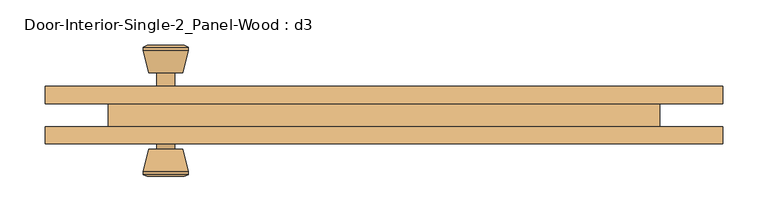
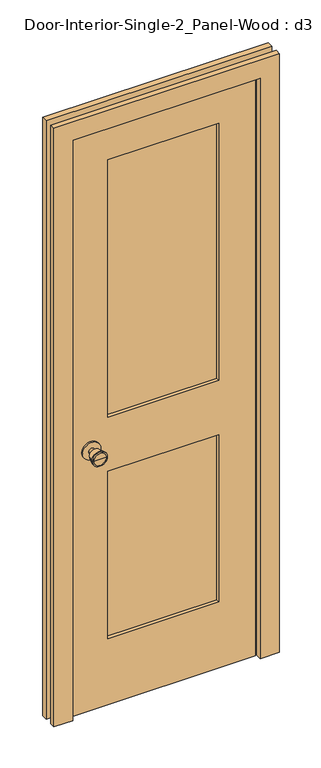
"""IFC4 building model written with IfcOpenShell, lengths in millimetres: door geometry, Door-Interior-Single-2_Panel-Wood : d3."""

from ifc_helpers import new_model, si_unit, point, frame, frame_2d, origin, place, context, project, spatial, polyline, circle_curve, trimmed, segment, composite_curve, outline, extrude, source, transform, mapped, element, save
from ifc_brep_helpers import plane_surface, cylinder_surface, revolved_surface, advanced_brep


def door_interior_single_2_panel_wood_d3_c9a7c184(model_context):
    return source(origin(), model_context, "Body", "SolidModel", [
        advanced_brep(
        [(-241.3, 31.4, 914.4), (-251.3, 31.4, 914.4), (-231.3, 31.4, 914.4), (-220.8241324, 80.4, 914.4), (-261.7758676, 80.4, 914.4), (-241.3, 80.4, 914.4), (-216.3, 78.5721319, 914.4), (-266.3, 78.5721319, 914.4), (-216.3, 75.1084537, 914.4), (-266.3, 75.1084537, 914.4), (-222.663764, 50.4, 914.4), (-259.936236, 50.4, 914.4), (-231.3, 50.4, 914.4), (-251.3, 50.4, 914.4)],
        [
            (0, 1),
            (1, 2, circle_curve(frame((-241.3, 31.4, 914.4), z_axis=(0.0, -1.0, 0.0), x_axis=(-1.0, 0.0, 0.0)), 10.0)),
            (2, 0),
            (2, 1, circle_curve(frame((-241.3, 31.4, 914.4), z_axis=(0.0, -1.0, 0.0), x_axis=(-1.0, 0.0, 0.0)), 10.0)),
            (3, 4, circle_curve(frame((-241.3, 80.4, 914.4), z_axis=(0.0, 1.0, 0.0), x_axis=(-1.0, 0.0, 0.0)), 20.4758676)),
            (4, 5),
            (5, 3),
            (4, 3, circle_curve(frame((-241.3, 80.4, 914.4), z_axis=(0.0, 1.0, 0.0), x_axis=(-1.0, 0.0, 0.0)), 20.4758676)),
            (6, 7, circle_curve(frame((-241.3, 78.5721319, 914.4), z_axis=(0.0, 1.0, 0.0), x_axis=(-1.0, 0.0, 0.0)), 25.0)),
            (7, 4),
            (3, 6),
            (7, 6, circle_curve(frame((-241.3, 78.5721319, 914.4), z_axis=(0.0, 1.0, 0.0), x_axis=(-1.0, 0.0, 0.0)), 25.0)),
            (8, 9, circle_curve(frame((-241.3, 75.1084537, 914.4), z_axis=(0.0, 1.0, 0.0), x_axis=(-1.0, 0.0, 0.0)), 25.0)),
            (9, 7),
            (6, 8),
            (9, 8, circle_curve(frame((-241.3, 75.1084537, 914.4), z_axis=(0.0, 1.0, 0.0), x_axis=(-1.0, 0.0, 0.0)), 25.0)),
            (10, 11, circle_curve(frame((-241.3, 50.4, 914.4), z_axis=(0.0, 1.0, 0.0), x_axis=(-1.0, 0.0, 0.0)), 18.636236)),
            (11, 9),
            (8, 10),
            (11, 10, circle_curve(frame((-241.3, 50.4, 914.4), z_axis=(0.0, 1.0, 0.0), x_axis=(-1.0, 0.0, 0.0)), 18.636236)),
            (12, 13, circle_curve(frame((-241.3, 50.4, 914.4), z_axis=(0.0, 1.0, 0.0), x_axis=(-1.0, 0.0, 0.0)), 10.0)),
            (13, 11),
            (10, 12),
            (13, 12, circle_curve(frame((-241.3, 50.4, 914.4), z_axis=(0.0, 1.0, 0.0), x_axis=(-1.0, 0.0, 0.0)), 10.0)),
            (1, 13),
            (12, 2),
        ],
        [
            plane_surface(frame((-241.3, 31.4, 914.4), z_axis=(0.0, -1.0, 0.0), x_axis=(-1.0, 0.0, 0.0))),
            plane_surface(frame((-241.3, 80.4, 914.4), z_axis=(0.0, 1.0, 0.0), x_axis=(-1.0, 0.0, 0.0))),
            revolved_surface(polyline([(-261.7758676, 80.4, 914.4), (-266.3, 78.5721319, 914.4)]), (-241.3, 31.4, 914.4), (0.0, -1.0, 0.0)),
            cylinder_surface(frame((-241.3, 31.4, 914.4), z_axis=(0.0, -1.0, 0.0), x_axis=(-1.0, 0.0, 0.0)), 25.0),
            revolved_surface(polyline([(-266.3, 75.1084537, 914.4), (-259.936236, 50.4, 914.4)]), (-241.3, 31.4, 914.4), (0.0, -1.0, 0.0)),
            plane_surface(frame((-241.3, 50.4, 914.4), z_axis=(0.0, -1.0, 0.0), x_axis=(-1.0, 0.0, 0.0))),
            cylinder_surface(frame((-241.3, 31.4, 914.4), z_axis=(0.0, -1.0, 0.0), x_axis=(-1.0, 0.0, 0.0)), 10.0),
        ],
        [
            (0, [[1, 2, 3]]),
            (0, [[-3, 4, -1]]),
            (1, [[5, 6, 7]]),
            (1, [[8, -7, -6]]),
            (2, [[9, 10, -5, 11]]),
            (2, [[12, -11, -8, -10]]),
            (3, [[13, 14, -9, 15]]),
            (3, [[16, -15, -12, -14]]),
            (4, [[17, 18, -13, 19]]),
            (4, [[20, -19, -16, -18]]),
            (5, [[21, 22, -17, 23]]),
            (5, [[24, -23, -20, -22]]),
            (6, [[-2, 25, -21, 26]]),
            (6, [[-4, -26, -24, -25]]),
        ],
    ),
        extrude(outline(composite_curve([segment(trimmed(circle_curve(frame_2d((914.4, -241.3)), 30.0), [point((914.4, -271.3))], [point((914.4, -211.3))], False, "CARTESIAN"), True, "CONTINUOUS"), segment(trimmed(circle_curve(frame_2d((914.4, -241.3)), 30.0), [point((914.4, -211.3))], [point((914.4, -271.3))], False, "CARTESIAN"), True, "CONTINUOUS")], self_intersect=False)), frame((0.0, 25.4, 0.0), z_axis=(0.0, 1.0, 0.0), x_axis=(0.0, 0.0, 1.0)), (0.0, 0.0, 1.0), 6.0),
        advanced_brep(
        [(-241.3, -15.525, 914.4), (-231.3, -15.525, 914.4), (-251.3, -15.525, 914.4), (-220.8241324, -64.525, 914.4), (-241.3, -64.525, 914.4), (-261.7758676, -64.525, 914.4), (-216.3, -62.6971319, 914.4), (-266.3, -62.6971319, 914.4), (-216.3, -59.2334537, 914.4), (-266.3, -59.2334537, 914.4), (-222.663764, -34.525, 914.4), (-259.936236, -34.525, 914.4), (-231.3, -34.525, 914.4), (-251.3, -34.525, 914.4)],
        [
            (0, 1),
            (1, 2, circle_curve(frame((-241.3, -15.525, 914.4), z_axis=(0.0, 1.0, 0.0), x_axis=(-1.0, 0.0, 0.0)), 10.0)),
            (2, 0),
            (2, 1, circle_curve(frame((-241.3, -15.525, 914.4), z_axis=(0.0, 1.0, 0.0), x_axis=(-1.0, 0.0, 0.0)), 10.0)),
            (3, 4),
            (4, 5),
            (5, 3, circle_curve(frame((-241.3, -64.525, 914.4), z_axis=(0.0, -1.0, 0.0), x_axis=(-1.0, 0.0, 0.0)), 20.4758676)),
            (3, 5, circle_curve(frame((-241.3, -64.525, 914.4), z_axis=(0.0, -1.0, 0.0), x_axis=(-1.0, 0.0, 0.0)), 20.4758676)),
            (6, 3),
            (5, 7),
            (7, 6, circle_curve(frame((-241.3, -62.6971319, 914.4), z_axis=(0.0, -1.0, 0.0), x_axis=(-1.0, 0.0, 0.0)), 25.0)),
            (6, 7, circle_curve(frame((-241.3, -62.6971319, 914.4), z_axis=(0.0, -1.0, 0.0), x_axis=(-1.0, 0.0, 0.0)), 25.0)),
            (8, 6),
            (7, 9),
            (9, 8, circle_curve(frame((-241.3, -59.2334537, 914.4), z_axis=(0.0, -1.0, 0.0), x_axis=(-1.0, 0.0, 0.0)), 25.0)),
            (8, 9, circle_curve(frame((-241.3, -59.2334537, 914.4), z_axis=(0.0, -1.0, 0.0), x_axis=(-1.0, 0.0, 0.0)), 25.0)),
            (10, 8),
            (9, 11),
            (11, 10, circle_curve(frame((-241.3, -34.525, 914.4), z_axis=(0.0, -1.0, 0.0), x_axis=(-1.0, 0.0, 0.0)), 18.636236)),
            (10, 11, circle_curve(frame((-241.3, -34.525, 914.4), z_axis=(0.0, -1.0, 0.0), x_axis=(-1.0, 0.0, 0.0)), 18.636236)),
            (12, 10),
            (11, 13),
            (13, 12, circle_curve(frame((-241.3, -34.525, 914.4), z_axis=(0.0, -1.0, 0.0), x_axis=(-1.0, 0.0, 0.0)), 10.0)),
            (12, 13, circle_curve(frame((-241.3, -34.525, 914.4), z_axis=(0.0, -1.0, 0.0), x_axis=(-1.0, 0.0, 0.0)), 10.0)),
            (1, 12),
            (13, 2),
        ],
        [
            plane_surface(frame((-241.3, -15.525, 914.4), z_axis=(0.0, 1.0, 0.0), x_axis=(-1.0, 0.0, 0.0))),
            plane_surface(frame((-241.3, -64.525, 914.4), z_axis=(0.0, -1.0, 0.0), x_axis=(-1.0, 0.0, 0.0))),
            revolved_surface(polyline([(-261.7758676, -64.525, 914.4), (-266.3, -62.6971319, 914.4)]), (-241.3, -15.525, 914.4), (0.0, 1.0, 0.0)),
            cylinder_surface(frame((-241.3, -15.525, 914.4), z_axis=(0.0, 1.0, 0.0), x_axis=(-1.0, 0.0, 0.0)), 25.0),
            revolved_surface(polyline([(-266.3, -59.2334537, 914.4), (-259.936236, -34.525, 914.4)]), (-241.3, -15.525, 914.4), (0.0, 1.0, 0.0)),
            plane_surface(frame((-241.3, -34.525, 914.4), z_axis=(0.0, 1.0, 0.0), x_axis=(-1.0, 0.0, 0.0))),
            cylinder_surface(frame((-241.3, -15.525, 914.4), z_axis=(0.0, 1.0, 0.0), x_axis=(-1.0, 0.0, 0.0)), 10.0),
        ],
        [
            (0, [[1, 2, 3]]),
            (0, [[-3, 4, -1]]),
            (1, [[5, 6, 7]]),
            (1, [[-6, -5, 8]]),
            (2, [[9, -7, 10, 11]]),
            (2, [[-10, -8, -9, 12]]),
            (3, [[13, -11, 14, 15]]),
            (3, [[-14, -12, -13, 16]]),
            (4, [[17, -15, 18, 19]]),
            (4, [[-18, -16, -17, 20]]),
            (5, [[21, -19, 22, 23]]),
            (5, [[-22, -20, -21, 24]]),
            (6, [[25, -23, 26, -2]]),
            (6, [[-26, -24, -25, -4]]),
        ],
    ),
        extrude(outline(composite_curve([segment(trimmed(circle_curve(frame_2d((914.4, -241.3)), 30.0), [point((914.4, -271.3))], [point((914.4, -211.3))], False, "CARTESIAN"), True, "CONTINUOUS"), segment(trimmed(circle_curve(frame_2d((914.4, -241.3)), 30.0), [point((914.4, -211.3))], [point((914.4, -271.3))], False, "CARTESIAN"), True, "CONTINUOUS")], self_intersect=False)), frame((0.0, -15.525, 0.0), z_axis=(0.0, 1.0, 0.0), x_axis=(0.0, 0.0, 1.0)), (0.0, 0.0, 1.0), 6.0),
        extrude(outline(polyline([(2032.0, -304.8), (0.0, -304.8), (0.0, 304.8), (2032.0, 304.8), (2032.0, -304.8)]), holes=[polyline([(1912.9375, -184.15), (1912.9375, 184.15), (1009.65, 184.15), (1009.65, -184.15), (1912.9375, -184.15)]), polyline([(819.15, -184.15), (819.15, 184.15), (231.775, 184.15), (231.775, -184.15), (819.15, -184.15)])]), frame((0.0, -9.525, 0.0), z_axis=(0.0, 1.0, 0.0), x_axis=(0.0, 0.0, 1.0)), (0.0, 0.0, 1.0), 34.925),
        extrude(outline(polyline([(184.15, 13.7583333), (184.15, 2.1166667), (-184.15, 2.1166667), (-184.15, 13.7583333), (184.15, 13.7583333)])), frame((0.0, 0.0, 1009.65), z_axis=(0.0, 0.0, 1.0), x_axis=(1.0, 0.0, 0.0)), (0.0, 0.0, 1.0), 903.2875),
        extrude(outline(polyline([(184.15, 13.7583333), (184.15, 2.1166667), (-184.15, 2.1166667), (-184.15, 13.7583333), (184.15, 13.7583333)])), frame((0.0, 0.0, 231.775), z_axis=(0.0, 0.0, 1.0), x_axis=(1.0, 0.0, 0.0)), (0.0, 0.0, 1.0), 587.375),
        extrude(outline(polyline([(0.0, 374.65), (2101.85, 374.65), (2101.85, -374.65), (0.0, -374.65), (0.0, -311.15), (2038.35, -311.15), (2038.35, 311.15), (0.0, 311.15), (0.0, 374.65)])), frame((0.0, -28.575, 0.0), z_axis=(0.0, 1.0, 0.0), x_axis=(0.0, 0.0, 1.0)), (0.0, 0.0, 1.0), 19.05),
        extrude(outline(polyline([(0.0, 374.65), (2101.85, 374.65), (2101.85, -374.65), (0.0, -374.65), (0.0, -311.15), (2038.35, -311.15), (2038.35, 311.15), (0.0, 311.15), (0.0, 374.65)])), frame((0.0, 15.875, 0.0), z_axis=(0.0, 1.0, 0.0), x_axis=(0.0, 0.0, 1.0)), (0.0, 0.0, 1.0), 19.05),
    ])


if __name__ == "__main__":
    model = new_model("IFC4")
    model_context = context("Model", 3, world=origin())
    ifc_project = project(units=[si_unit("LENGTHUNIT", "METRE", prefix="MILLI")], contexts=[model_context])
    site = spatial("IfcSite", under=ifc_project)
    building = spatial("IfcBuilding", under=site)
    placement = place(None, origin())
    door_interior_single_2_panel_wood_d3_shape = door_interior_single_2_panel_wood_d3_c9a7c184(model_context)
    element("IfcDoor", 1, ObjectType="Door-Interior-Single-2_Panel-Wood : d3", at=placement, inside=building, context=model_context, shape_type="MappedRepresentation", body=[
        mapped(door_interior_single_2_panel_wood_d3_shape, transform((0.0, 0.0, 0.0), x_axis=(1.0, 0.0, 0.0), y_axis=(0.0, 1.0, 0.0), z_axis=(0.0, 0.0, 1.0))),
    ])
    save(model, "model.ifc")

# Revit data of these elements
# Type "Door-Interior-Single-2_Panel-Wood : d3"
#   Type Mark = "13"
#   Assembly Code = "C1020300"
#   Analytic Construction = "Wooden"
#   Top Rail = 0' - 4 11/16"
#   Thickness = 0' - 1 3/8"
#   Thermal Resistance (R) = 2.5876 (h·ft²·°F)/BTU
#   Swing Angle [instance default] = 90.00°
#   Stiles = 0' - 4 3/4"
#   Rough Width = 2' - 2"
#   Rough Height = 6' - 9"
#   Lock Rail = 0' - 7 1/2"
#   Height = 6' - 8"
#   Width = 2' - 0"
#   Heat Transfer Coefficient (U) = 0.3865 BTU/(h·ft²·°F)
#   Bottom Rail = 0' - 9 1/8"
#   Trim Material = Cherry
#   Panel Material = Cherry
#   Frame Material = Cherry
#   Door Handle Material = Aluminum
#   Visual Light Transmittance = 0
#   Solar Heat Gain Coefficient = 0
#   Wall Closure = (empty or 0)
#   Function = (empty or 0)
# Element 1 (IfcDoor, "Door-Interior-Single-2_Panel-Wood : d3")
#   Materials on its faces: "Cherry", "Aluminum"
# Materials
#   "Cherry": class "Wood", colour RGB 226 177 128, transparency 0, Description = "Prunus Serotina", Cost = 0
#   "Aluminum": class "Metal", colour RGB 247 247 247, transparency 0, Description = "Aluminum 6061", Cost = 0
